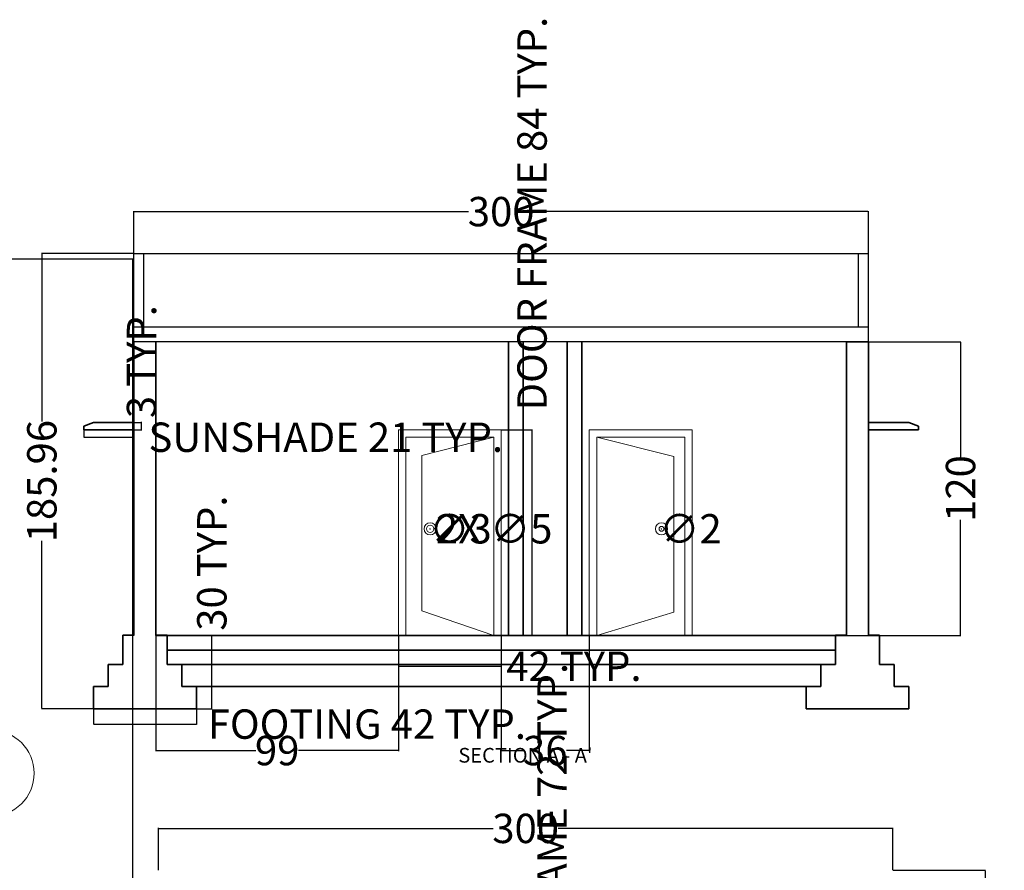
# Model space of a CAD drawing. Units: inches. Extents: x -101 to 786, y 26 to 880.
# Tile 9 of 9: x 379 to 781, y 532 to 879. Entities that reach past the tile are written whole.
import ezdxf

# ---------------------------------------------------------------- set-up
doc = ezdxf.new("R2010")
doc.units = ezdxf.units.IN
doc.header["$MEASUREMENT"] = 0
for name, color, linetype, lineweight in [('A-ANNO-DIMS', 2, 'Continuous', 18), ('A-ANNO-SYMB', 2, 'Continuous', 18), ('A-ANNO-TEXT', 7, 'Continuous', 25), ('A-DOOR', 4, 'Continuous', 20), ('A-ROOF', 7, 'Continuous', 30), ('A-SECT', 7, 'Continuous', 35), ('S-FNDN', 7, 'Continuous', 35)]:
    doc.layers.add(name, color=color, linetype=linetype, lineweight=lineweight)
doc.styles.get("Standard").update_dxf_attribs({"font": 'arial.ttf'})
doc.dimstyles.get("Standard").update_dxf_attribs({"dimtxt": 12, "dimasz": 0.18, "dimexe": 0.18, "dimexo": 0.0625, "dimgap": 0.09, "dimtad": 0, "dimdec": 1, "dimzin": 0, "dimdsep": 46, "dimlunit": 3, "dimtxsty": 'Standard', "dimcen": 0.09, "dimadec": 0, "dimazin": 0, "dimtfac": 1, "dimtdec": 1, "dimtofl": 0, "dimtmove": 0, "dimatfit": 3, "dimfxl": 1, "dimtolj": 1, "dimtzin": 0, "dimarcsym": 0})

# ---------------------------------------------------------------- blocks, each defined once
blk = doc.blocks.new('SUNSHADE-SECTION')
for p, q in [((0, 1.5), (4, 3)), ((0, 0), (0, 1.5)), ((20.5, 3), (4, 3)), ((4, 0), (0, 0)), ((20.5, 0), (4, 0))]:
    blk.add_line(p, q)
blk = doc.blocks.new('FOOTING-STEPPED-42')
for p, q in [((12, 30), (12, 18)), ((16.5, 30), (12, 30)), ((30, 30), (25.5, 30)), ((30, 18), (30, 30)), ((12, 18), (6, 18)), ((6, 18), (6, 9)), ((36, 18), (30, 18)), ((36, 9), (36, 18)), ((6, 9), (0, 9)), ((0, 9), (0, 0)), ((42, 9), (36, 9)), ((42, 0), (42, 9)), ((0, 0), (42, 0))]:
    blk.add_line(p, q)
blk = doc.blocks.new('DOOR-FRAME-36x84-SECT')
blk.add_line((0, 84), (42, 84))
for points in [[(42, 0), (42, 84), (0, 84), (0, 0)], [(39, 0), (39, 81), (3, 81), (3, 0)]]:
    blk.add_lwpolyline(points)
blk = doc.blocks.new('*D45')
at = {"layer": 'A-ANNO-DIMS', "color": 0, "lineweight": -2, "transparency": 16777216}
for p, q in [((404.81, 711.9), (404.81, 708.7)), ((425.31, 711.9), (425.31, 708.7)), ((404.99, 708.88), (425.13, 708.88)), ((425.31, 708.88), (425.49, 708.88))]:
    blk.add_line(p, q, dxfattribs=at)
at = {"layer": 'A-ANNO-DIMS', "color": 0, "transparency": 16777216}
for points in [[(404.99, 708.91), (404.99, 708.85), (404.81, 708.88)], [(425.13, 708.91), (425.13, 708.85), (425.31, 708.88)]]:
    blk.add_solid(points, dxfattribs=at)
at = {"layer": 'Defpoints', "color": 0, "transparency": 16777216}
for p in [(404.81, 711.96), (425.31, 711.96), (425.31, 708.88)]:
    blk.add_point(p, dxfattribs=at)
at = {"layer": 'A-ANNO-DIMS', "color": 0, "transparency": 16777216, "insert": (503.66, 708.88), "char_height": 12, "attachment_point": 5}
blk.add_mtext('\\A1;SUNSHADE 21 TYP.', dxfattribs=at)
blk = doc.blocks.new('*D46')
at = {"layer": 'A-ANNO-DIMS', "color": 0, "lineweight": -2, "transparency": 16777216}
for p, q in [((425.37, 714.96), (428.57, 714.96)), ((425.37, 711.96), (428.57, 711.96)), ((428.39, 714.96), (428.39, 715.14)), ((428.39, 712.14), (428.39, 714.78))]:
    blk.add_line(p, q, dxfattribs=at)
at = {"layer": 'A-ANNO-DIMS', "color": 0, "transparency": 16777216}
for points in [[(428.36, 714.78), (428.42, 714.78), (428.39, 714.96)], [(428.36, 712.14), (428.42, 712.14), (428.39, 711.96)]]:
    blk.add_solid(points, dxfattribs=at)
at = {"layer": 'Defpoints', "color": 0, "transparency": 16777216}
for p in [(425.31, 714.96), (425.31, 711.96), (428.39, 714.96)]:
    blk.add_point(p, dxfattribs=at)
at = {"layer": 'A-ANNO-DIMS', "color": 0, "transparency": 16777216, "insert": (428.39, 739.77), "char_height": 12, "attachment_point": 5, "rotation": 90}
blk.add_mtext('\\A1;3 TYP.', dxfattribs=at)
blk = doc.blocks.new('*D53')
at = {"layer": 'A-ANNO-DIMS', "color": 0, "lineweight": -2, "transparency": 16777216}
for p, q in [((408.81, 597.9), (408.81, 591.48)), ((450.81, 597.9), (450.81, 591.48)), ((408.99, 591.66), (450.63, 591.66)), ((450.81, 591.66), (450.99, 591.66))]:
    blk.add_line(p, q, dxfattribs=at)
at = {"layer": 'A-ANNO-DIMS', "color": 0, "transparency": 16777216}
for points in [[(408.99, 591.69), (408.99, 591.63), (408.81, 591.66)], [(450.63, 591.69), (450.63, 591.63), (450.81, 591.66)]]:
    blk.add_solid(points, dxfattribs=at)
at = {"layer": 'Defpoints', "color": 0, "transparency": 16777216}
for p in [(408.81, 597.96), (450.81, 597.96), (450.81, 591.66)]:
    blk.add_point(p, dxfattribs=at)
at = {"layer": 'A-ANNO-DIMS', "color": 0, "transparency": 16777216, "insert": (520.45, 591.66), "char_height": 12, "attachment_point": 5}
blk.add_mtext('\\A1;FOOTING 42 TYP.', dxfattribs=at)
blk = doc.blocks.new('*D54')
at = {"layer": 'A-ANNO-DIMS', "color": 0, "lineweight": -2, "transparency": 16777216}
for p, q in [((450.87, 627.96), (457.29, 627.96)), ((457.11, 627.96), (457.11, 628.14)), ((457.11, 598.14), (457.11, 627.78)), ((450.87, 597.96), (457.29, 597.96))]:
    blk.add_line(p, q, dxfattribs=at)
at = {"layer": 'A-ANNO-DIMS', "color": 0, "transparency": 16777216}
for points in [[(457.08, 627.78), (457.14, 627.78), (457.11, 627.96)], [(457.08, 598.14), (457.14, 598.14), (457.11, 597.96)]]:
    blk.add_solid(points, dxfattribs=at)
at = {"layer": 'Defpoints', "color": 0, "transparency": 16777216}
for p in [(450.81, 627.96), (457.11, 627.96), (450.81, 597.96)]:
    blk.add_point(p, dxfattribs=at)
at = {"layer": 'A-ANNO-DIMS', "color": 0, "transparency": 16777216, "insert": (457.11, 657.43), "char_height": 12, "attachment_point": 5, "rotation": 90}
blk.add_mtext('\\A1;30 TYP.', dxfattribs=at)
blk = doc.blocks.new('*D61')
at = {"layer": 'A-ANNO-DIMS', "color": 0, "lineweight": -2, "transparency": 16777216}
for p, q in [((575.37, 711.92), (588.09, 711.92)), ((587.91, 711.92), (587.91, 712.1)), ((587.91, 628.1), (587.91, 711.74)), ((575.37, 627.92), (588.09, 627.92))]:
    blk.add_line(p, q, dxfattribs=at)
at = {"layer": 'A-ANNO-DIMS', "color": 0, "transparency": 16777216}
for points in [[(587.88, 711.74), (587.94, 711.74), (587.91, 711.92)], [(587.88, 628.1), (587.94, 628.1), (587.91, 627.92)]]:
    blk.add_solid(points, dxfattribs=at)
at = {"layer": 'Defpoints', "color": 0, "transparency": 16777216}
for p in [(575.31, 711.92), (587.91, 711.92), (575.31, 627.92)]:
    blk.add_point(p, dxfattribs=at)
at = {"layer": 'A-ANNO-DIMS', "color": 0, "transparency": 16777216, "insert": (587.91, 800.24), "char_height": 12, "attachment_point": 5, "rotation": 90}
blk.add_mtext('\\A1;DOOR FRAME 84 TYP.', dxfattribs=at)
blk = doc.blocks.new('*D62')
at = {"layer": 'A-ANNO-DIMS', "color": 0, "lineweight": -2, "transparency": 16777216}
for p, q in [((533.31, 627.86), (533.31, 615.14)), ((575.31, 627.86), (575.31, 615.14)), ((533.49, 615.32), (575.13, 615.32)), ((575.31, 615.32), (575.49, 615.32))]:
    blk.add_line(p, q, dxfattribs=at)
at = {"layer": 'A-ANNO-DIMS', "color": 0, "transparency": 16777216}
for points in [[(533.49, 615.35), (533.49, 615.29), (533.31, 615.32)], [(575.13, 615.35), (575.13, 615.29), (575.31, 615.32)]]:
    blk.add_solid(points, dxfattribs=at)
at = {"layer": 'Defpoints', "color": 0, "transparency": 16777216}
for p in [(533.31, 627.92), (575.31, 627.92), (575.31, 615.32)]:
    blk.add_point(p, dxfattribs=at)
at = {"layer": 'A-ANNO-DIMS', "color": 0, "transparency": 16777216, "insert": (605.03, 615.32), "char_height": 12, "attachment_point": 5}
blk.add_mtext('\\A1;42 TYP.', dxfattribs=at)
blk = doc.blocks.new('*D63')
at = {"layer": 'A-ANNO-DIMS', "color": 0, "lineweight": -2, "transparency": 16777216}
for p, q in [((585.37, 447.92), (596.29, 447.92)), ((596.11, 447.92), (596.11, 448.1)), ((596.11, 376.1), (596.11, 447.74)), ((585.37, 375.92), (596.29, 375.92))]:
    blk.add_line(p, q, dxfattribs=at)
at = {"layer": 'A-ANNO-DIMS', "color": 0, "transparency": 16777216}
for points in [[(596.08, 447.74), (596.14, 447.74), (596.11, 447.92)], [(596.08, 376.1), (596.14, 376.1), (596.11, 375.92)]]:
    blk.add_solid(points, dxfattribs=at)
at = {"layer": 'Defpoints', "color": 0, "transparency": 16777216}
for p in [(585.31, 447.92), (596.11, 447.92), (585.31, 375.92)]:
    blk.add_point(p, dxfattribs=at)
at = {"layer": 'A-ANNO-DIMS', "color": 0, "transparency": 16777216, "insert": (596.11, 536.24), "char_height": 12, "attachment_point": 5, "rotation": 90}
blk.add_mtext('\\A1;DOOR FRAME 72 TYP.', dxfattribs=at)
blk = doc.blocks.new('*D80')
at = {"layer": 'A-ANNO-DIMS', "color": 0, "lineweight": -2, "transparency": 16777216}
for p, q in [((323.57, 781.8), (424.94, 781.8)), ((424.76, 781.62), (424.76, 472.49)), ((424.76, 122.52), (424.76, 431.66)), ((323.57, 122.34), (424.94, 122.34))]:
    blk.add_line(p, q, dxfattribs=at)
at = {"layer": 'A-ANNO-DIMS', "color": 0, "transparency": 16777216}
for points in [[(424.73, 781.62), (424.79, 781.62), (424.76, 781.8)], [(424.73, 122.52), (424.79, 122.52), (424.76, 122.34)]]:
    blk.add_solid(points, dxfattribs=at)
at = {"layer": 'Defpoints', "color": 0, "transparency": 16777216}
for p in [(323.51, 781.8), (424.76, 781.8), (323.51, 122.34)]:
    blk.add_point(p, dxfattribs=at)
at = {"layer": 'A-ANNO-DIMS', "color": 0, "transparency": 16777216, "insert": (424.76, 452.07), "char_height": 12, "attachment_point": 5, "rotation": 90}
blk.add_mtext('\\A1;659.5', dxfattribs=at)
blk = doc.blocks.new('*D119')
at = {"layer": 'A-ANNO-DIMS', "color": 0, "lineweight": -2, "transparency": 16777216}
for p, q in [((425.31, 783.99), (425.31, 801.23)), ((425.49, 801.05), (561.99, 801.05)), ((725.13, 801.05), (588.63, 801.05)), ((725.31, 783.99), (725.31, 801.23))]:
    blk.add_line(p, q, dxfattribs=at)
at = {"layer": 'A-ANNO-DIMS', "color": 0, "transparency": 16777216}
for points in [[(425.49, 801.08), (425.49, 801.02), (425.31, 801.05)], [(725.13, 801.08), (725.13, 801.02), (725.31, 801.05)]]:
    blk.add_solid(points, dxfattribs=at)
at = {"layer": 'Defpoints', "color": 0, "transparency": 16777216}
for p in [(725.31, 801.05), (425.31, 783.92), (725.31, 783.92)]:
    blk.add_point(p, dxfattribs=at)
at = {"layer": 'A-ANNO-DIMS', "color": 0, "transparency": 16777216, "insert": (575.31, 801.05), "char_height": 12, "attachment_point": 5}
blk.add_mtext('\\A1;300', dxfattribs=at)
blk = doc.blocks.new('*D120')
at = {"layer": 'A-ANNO-DIMS', "color": 0, "lineweight": -2, "transparency": 16777216}
for p, q in [((425.25, 783.92), (387.5, 783.92)), ((387.68, 783.74), (387.68, 715.37)), ((387.68, 598.14), (387.68, 666.51)), ((408.74, 597.96), (387.5, 597.96))]:
    blk.add_line(p, q, dxfattribs=at)
at = {"layer": 'A-ANNO-DIMS', "color": 0, "transparency": 16777216}
for points in [[(387.65, 783.74), (387.71, 783.74), (387.68, 783.92)], [(387.65, 598.14), (387.71, 598.14), (387.68, 597.96)]]:
    blk.add_solid(points, dxfattribs=at)
at = {"layer": 'Defpoints', "color": 0, "transparency": 16777216}
for p in [(387.68, 783.92), (425.31, 783.92), (408.81, 597.96)]:
    blk.add_point(p, dxfattribs=at)
at = {"layer": 'A-ANNO-DIMS', "color": 0, "transparency": 16777216, "insert": (387.68, 690.94), "char_height": 12, "attachment_point": 5, "rotation": 90}
blk.add_mtext('\\A1;185.96', dxfattribs=at)
blk = doc.blocks.new('*D121')
at = {"layer": 'A-ANNO-DIMS', "color": 0, "lineweight": -2, "transparency": 16777216}
for p, q in [((716.37, 747.92), (763.12, 747.92)), ((762.94, 747.74), (762.94, 700.69)), ((762.94, 628.1), (762.94, 675.16)), ((716.37, 627.92), (763.12, 627.92))]:
    blk.add_line(p, q, dxfattribs=at)
at = {"layer": 'A-ANNO-DIMS', "color": 0, "transparency": 16777216}
for points in [[(762.91, 747.74), (762.97, 747.74), (762.94, 747.92)], [(762.91, 628.1), (762.97, 628.1), (762.94, 627.92)]]:
    blk.add_solid(points, dxfattribs=at)
at = {"layer": 'Defpoints', "color": 0, "transparency": 16777216}
for p in [(716.31, 747.92), (762.94, 747.92), (716.31, 627.92)]:
    blk.add_point(p, dxfattribs=at)
at = {"layer": 'A-ANNO-DIMS', "color": 0, "transparency": 16777216, "insert": (762.94, 687.92), "char_height": 12, "attachment_point": 5, "rotation": 90}
blk.add_mtext('\\A1;120', dxfattribs=at)
blk = doc.blocks.new('*D122')
at = {"layer": 'A-ANNO-DIMS', "color": 0, "lineweight": -2, "transparency": 16777216}
for p, q in [((434.31, 627.86), (434.31, 580.66)), ((533.31, 627.86), (533.31, 580.66)), ((434.49, 580.84), (475.11, 580.84)), ((533.13, 580.84), (492.51, 580.84))]:
    blk.add_line(p, q, dxfattribs=at)
at = {"layer": 'A-ANNO-DIMS', "color": 0, "transparency": 16777216}
for points in [[(434.49, 580.87), (434.49, 580.81), (434.31, 580.84)], [(533.13, 580.87), (533.13, 580.81), (533.31, 580.84)]]:
    blk.add_solid(points, dxfattribs=at)
at = {"layer": 'Defpoints', "color": 0, "transparency": 16777216}
for p in [(434.31, 627.92), (533.31, 627.92), (533.31, 580.84)]:
    blk.add_point(p, dxfattribs=at)
at = {"layer": 'A-ANNO-DIMS', "color": 0, "transparency": 16777216, "insert": (483.81, 580.84), "char_height": 12, "attachment_point": 5}
blk.add_mtext('\\A1;99', dxfattribs=at)
blk = doc.blocks.new('*D123')
at = {"layer": 'A-ANNO-DIMS', "color": 0, "lineweight": -2, "transparency": 16777216}
for p, q in [((575.31, 627.86), (575.31, 580.66)), ((611.31, 627.86), (611.31, 580.66)), ((575.49, 580.84), (584.64, 580.84)), ((611.13, 580.84), (601.99, 580.84))]:
    blk.add_line(p, q, dxfattribs=at)
at = {"layer": 'A-ANNO-DIMS', "color": 0, "transparency": 16777216}
for points in [[(575.49, 580.87), (575.49, 580.81), (575.31, 580.84)], [(611.13, 580.87), (611.13, 580.81), (611.31, 580.84)]]:
    blk.add_solid(points, dxfattribs=at)
at = {"layer": 'Defpoints', "color": 0, "transparency": 16777216}
for p in [(575.31, 627.92), (611.31, 627.92), (611.31, 580.84)]:
    blk.add_point(p, dxfattribs=at)
at = {"layer": 'A-ANNO-DIMS', "color": 0, "transparency": 16777216, "insert": (593.31, 580.84), "char_height": 12, "attachment_point": 5}
blk.add_mtext('\\A1;36', dxfattribs=at)
blk = doc.blocks.new('*D124')
at = {"layer": 'A-ANNO-DIMS', "color": 0, "lineweight": -2, "transparency": 16777216}
for p, q in [((435.31, 531.99), (435.31, 549.23)), ((435.49, 549.05), (571.99, 549.05)), ((735.13, 549.05), (598.63, 549.05)), ((735.31, 531.99), (735.31, 549.23))]:
    blk.add_line(p, q, dxfattribs=at)
at = {"layer": 'A-ANNO-DIMS', "color": 0, "transparency": 16777216}
for points in [[(435.49, 549.08), (435.49, 549.02), (435.31, 549.05)], [(735.13, 549.08), (735.13, 549.02), (735.31, 549.05)]]:
    blk.add_solid(points, dxfattribs=at)
at = {"layer": 'Defpoints', "color": 0, "transparency": 16777216}
for p in [(735.31, 549.05), (435.31, 531.92), (735.31, 531.92)]:
    blk.add_point(p, dxfattribs=at)
at = {"layer": 'A-ANNO-DIMS', "color": 0, "transparency": 16777216, "insert": (585.31, 549.05), "char_height": 12, "attachment_point": 5}
blk.add_mtext('\\A1;300', dxfattribs=at)
blk = doc.blocks.new('*D125')
at = {"layer": 'A-ANNO-DIMS', "color": 0, "lineweight": -2, "transparency": 16777216}
for p, q in [((735.37, 531.92), (773.12, 531.92)), ((772.94, 531.74), (772.94, 463.37)), ((772.94, 346.14), (772.94, 414.51)), ((751.88, 345.96), (773.12, 345.96))]:
    blk.add_line(p, q, dxfattribs=at)
at = {"layer": 'A-ANNO-DIMS', "color": 0, "transparency": 16777216}
for points in [[(772.91, 531.74), (772.97, 531.74), (772.94, 531.92)], [(772.91, 346.14), (772.97, 346.14), (772.94, 345.96)]]:
    blk.add_solid(points, dxfattribs=at)
at = {"layer": 'Defpoints', "color": 0, "transparency": 16777216}
for p in [(735.31, 531.92), (772.94, 531.92), (751.82, 345.96)]:
    blk.add_point(p, dxfattribs=at)
at = {"layer": 'A-ANNO-DIMS', "color": 0, "transparency": 16777216, "insert": (772.94, 438.94), "char_height": 12, "attachment_point": 5, "rotation": 90}
blk.add_mtext('\\A1;185.96', dxfattribs=at)
blk = doc.blocks.new('*D136')
at = {"layer": 'A-ANNO-DIMS', "color": 0, "lineweight": -2, "transparency": 16777216}
for p, q in [((546.22, 671.46), (546.4, 671.46)), ((546.31, 671.37), (546.31, 671.55)), ((549.17, 671.46), (548.99, 671.46))]:
    blk.add_line(p, q, dxfattribs=at)
at = {"layer": 'A-ANNO-DIMS', "color": 0, "transparency": 16777216}
blk.add_solid([(548.99, 671.49), (548.99, 671.43), (548.81, 671.46)], dxfattribs=at)
at = {"layer": 'Defpoints', "color": 0, "transparency": 16777216}
for p in [(543.81, 671.46), (548.81, 671.46)]:
    blk.add_point(p, dxfattribs=at)
at = {"layer": 'A-ANNO-DIMS', "color": 0, "transparency": 16777216, "insert": (572.44, 671.46), "char_height": 12, "attachment_point": 5, "rotation": 0.0081}
blk.add_mtext('\\A1;2X ∅5', dxfattribs=at)
blk = doc.blocks.new('*D137')
at = {"layer": 'A-ANNO-DIMS', "color": 0, "lineweight": -2, "transparency": 16777216}
for p, q in [((546.22, 671.46), (546.4, 671.46)), ((546.31, 671.37), (546.31, 671.55)), ((548.17, 671.46), (547.99, 671.46))]:
    blk.add_line(p, q, dxfattribs=at)
at = {"layer": 'A-ANNO-DIMS', "color": 0, "transparency": 16777216}
blk.add_solid([(547.99, 671.49), (547.99, 671.43), (547.81, 671.46)], dxfattribs=at)
at = {"layer": 'Defpoints', "color": 0, "transparency": 16777216}
for p in [(544.81, 671.46), (547.81, 671.46)]:
    blk.add_point(p, dxfattribs=at)
at = {"layer": 'A-ANNO-DIMS', "color": 0, "transparency": 16777216, "insert": (558.72, 671.46), "char_height": 12, "attachment_point": 5, "rotation": 0.0136}
blk.add_mtext('\\A1;∅3', dxfattribs=at)
blk = doc.blocks.new('*D138')
at = {"layer": 'A-ANNO-DIMS', "color": 0, "lineweight": -2, "transparency": 16777216}
for p, q in [((640.72, 671.46), (640.9, 671.46)), ((640.81, 671.37), (640.81, 671.55)), ((642.17, 671.46), (641.99, 671.46))]:
    blk.add_line(p, q, dxfattribs=at)
at = {"layer": 'A-ANNO-DIMS', "color": 0, "transparency": 16777216}
blk.add_solid([(641.99, 671.49), (641.99, 671.43), (641.81, 671.46)], dxfattribs=at)
at = {"layer": 'Defpoints', "color": 0, "transparency": 16777216}
for p in [(639.81, 671.46), (641.81, 671.46)]:
    blk.add_point(p, dxfattribs=at)
at = {"layer": 'A-ANNO-DIMS', "color": 0, "transparency": 16777216, "insert": (652.66, 671.46), "char_height": 12, "attachment_point": 5, "rotation": 0.0203}
blk.add_mtext('\\A1;∅2', dxfattribs=at)

msp = doc.modelspace()

# ---------------------------------------------------------------- linework, layer by layer
at = {"layer": 'A-ANNO-SYMB'}
msp.add_circle((366.8306, 571.5872), 17.6773, dxfattribs=at)
at = {"layer": 'A-DOOR'}
for p, q in [((572.3117, 708.9238), (542.8583, 701.3432)), ((614.3117, 708.9238), (645.8069, 700.9606)), ((542.8583, 701.3432), (542.8583, 637.9606)), ((645.8069, 700.9606), (645.8069, 637.4606)), ((542.8583, 637.9606), (572.3117, 627.9238)), ((645.8069, 637.4606), (614.3117, 627.9238))]:
    msp.add_line(p, q, dxfattribs=at)
for centre, radius in [((546.3069, 671.4606), 2.5), ((546.3069, 671.4606), 1.5), ((640.8069, 671.4606), 2.5), ((640.8069, 671.4606), 2.5), ((640.8069, 671.4606), 2.5), ((640.8069, 671.4606), 2.5), ((640.8069, 671.4606), 1)]:
    msp.add_circle(centre, radius, dxfattribs=at)
at = {"layer": 'A-ROOF'}
for p, q in [((425.3117, 783.9238), (725.3117, 783.9238)), ((425.3117, 747.9238), (425.3117, 783.9238)), ((429.3117, 753.9238), (429.3117, 783.9238)), ((721.3117, 753.9238), (721.3117, 783.9238)), ((725.3117, 747.9238), (725.3117, 783.9238)), ((425.3117, 753.9238), (725.3117, 753.9238)), ((425.3117, 747.9238), (725.3117, 747.9238))]:
    msp.add_line(p, q, dxfattribs=at)
at = {"layer": 'A-SECT'}
for p, q in [((425.3117, 627.9238), (425.3117, 747.9238)), ((434.3117, 627.9238), (434.3117, 747.9238)), ((578.3117, 627.9238), (578.3117, 747.9238)), ((584.3117, 627.9238), (584.3117, 747.9238)), ((602.3117, 627.9238), (602.3117, 747.9238)), ((608.3117, 627.9238), (608.3117, 747.9238)), ((716.3117, 627.9238), (716.3117, 747.9238)), ((725.3117, 627.9238), (725.3117, 747.9238)), ((434.3117, 627.9238), (716.3117, 627.9238))]:
    msp.add_line(p, q, dxfattribs=at)
at = {"layer": 'S-FNDN'}
for p, q in [((438.8069, 621.9238), (711.8166, 621.9238)), ((444.8069, 615.9606), (705.8166, 615.9606)), ((450.8069, 606.9606), (699.8166, 606.9606))]:
    msp.add_line(p, q, dxfattribs=at)

# ---------------------------------------------------------------- block references
at = {"layer": 'A-DOOR'}
for p in [(533.312, 627.924), (611.312, 627.924)]:
    msp.add_blockref('DOOR-FRAME-36x84-SECT', p, dxfattribs=at)
at = {"layer": 'A-SECT'}
msp.add_blockref('SUNSHADE-SECTION', (404.807, 711.961), dxfattribs=at)
at = {"layer": 'A-SECT', "extrusion": (0, 0, -1), "zscale": -1}
msp.add_blockref('SUNSHADE-SECTION', (-745.8165, 711.961), dxfattribs=at)
at = {"layer": 'S-FNDN'}
msp.add_blockref('FOOTING-STEPPED-42', (408.807, 597.961), dxfattribs=at)
at = {"layer": 'S-FNDN', "extrusion": (0, 0, -1), "zscale": -1}
msp.add_blockref('FOOTING-STEPPED-42', (-741.8165, 597.961), dxfattribs=at)

# ---------------------------------------------------------------- texts
at = {"layer": 'A-ANNO-TEXT'}
msp.add_text("SECTION A - A'", height=6, dxfattribs=at).set_placement((557.8117, 575.9238))

# ---------------------------------------------------------------- dimensions: what is measured, and where the dimension line sits
at = {"layer": 'A-ANNO-DIMS'}
for base, p1, p2, text, picture, middle in [((587.9117, 711.9238), (575.3117, 627.9238), (575.3117, 711.9238), 'DOOR FRAME <> TYP.', '*D61', (587.9117, 800.2415)), ((428.3875, 714.9606), (425.3117, 711.9606), (425.3117, 714.9606), '<> TYP.', '*D46', (428.3875, 739.7709)), ((457.1069, 627.9606), (450.8069, 597.9606), (450.8069, 627.9606), '<> TYP.', '*D54', (457.1069, 657.4326)), ((596.1117, 447.9238), (585.3117, 375.9238), (585.3117, 447.9238), 'DOOR FRAME <> TYP.', '*D63', (596.1117, 536.2415))]:
    dim = msp.add_linear_dim(base=base, p1=p1, p2=p2, angle=90, text=text, dimstyle='Standard', override={"dimdec": 0, "dimlfac": 1, "dimrnd": 0, "dimzin": 0, "dimdsep": 46, "dimlunit": 2}, dxfattribs=at)
    dim.commit()
    dim.dimension.update_dxf_attribs({"geometry": picture, "text_midpoint": middle})
for base, p1, p2, picture, middle in [((725.3117, 801.0488), (425.3117, 783.9238), (725.3117, 783.9238), '*D119', (575.3117, 801.0488)), ((533.3117, 580.8356), (434.3117, 627.9238), (533.3117, 627.9238), '*D122', (483.8117, 580.8356)), ((611.3117, 580.8356), (575.3117, 627.9238), (611.3117, 627.9238), '*D123', (593.3117, 580.8356)), ((735.3117, 549.0488), (435.3117, 531.9238), (735.3117, 531.9238), '*D124', (585.3117, 549.0488))]:
    dim = msp.add_linear_dim(base=base, p1=p1, p2=p2, dimstyle='Standard', override={"dimdec": 0, "dimlfac": 1, "dimrnd": 0, "dimzin": 0, "dimdsep": 46, "dimlunit": 2}, dxfattribs=at)
    dim.commit()
    dim.dimension.update_dxf_attribs({"geometry": picture, "text_midpoint": middle})
for base, p1, p2, override, picture, middle in [((424.7579, 781.8033), (323.5071, 122.3446), (323.5071, 781.8033), {"dimdec": 1, "dimlfac": 1, "dimrnd": 0, "dimzin": 0, "dimdsep": 46, "dimlunit": 2}, '*D80', (424.7579, 452.0739)), ((387.6819, 783.9238), (408.8069, 597.9606), (425.3117, 783.9238), {"dimdec": 2, "dimlfac": 1, "dimrnd": 0, "dimzin": 0, "dimdsep": 46, "dimlunit": 2}, '*D120', (387.6819, 690.9422)), ((762.9416, 747.9238), (716.3117, 627.9238), (716.3117, 747.9238), {"dimdec": 0, "dimlfac": 1, "dimrnd": 0, "dimzin": 0, "dimdsep": 46, "dimlunit": 2}, '*D121', (762.9416, 687.9238)), ((772.9416, 531.9238), (751.8166, 345.9606), (735.3117, 531.9238), {"dimdec": 2, "dimlfac": 1, "dimrnd": 0, "dimzin": 0, "dimdsep": 46, "dimlunit": 2}, '*D125', (772.9416, 438.9422))]:
    dim = msp.add_linear_dim(base=base, p1=p1, p2=p2, angle=90, dimstyle='Standard', override=override, dxfattribs=at)
    dim.commit()
    dim.dimension.update_dxf_attribs({"geometry": picture, "text_midpoint": middle})
for base, p1, p2, text, picture, middle in [((425.3117, 708.8849), (404.8069, 711.9606), (425.3117, 711.9606), 'SUNSHADE <> TYP.', '*D45', (503.6636, 708.8849)), ((575.3117, 615.3238), (533.3117, 627.9238), (575.3117, 627.9238), '<> TYP.', '*D62', (605.0292, 615.3238)), ((450.8069, 591.6606), (408.8069, 597.9606), (450.8069, 597.9606), 'FOOTING <> TYP.', '*D53', (520.4534, 591.6606))]:
    dim = msp.add_linear_dim(base=base, p1=p1, p2=p2, text=text, dimstyle='Standard', override={"dimdec": 0, "dimlfac": 1, "dimrnd": 0, "dimzin": 0, "dimdsep": 46, "dimlunit": 2}, dxfattribs=at)
    dim.commit()
    dim.dimension.update_dxf_attribs({"geometry": picture, "text_midpoint": middle})
dim = msp.add_diameter_dim_2p(p1=(543.8069, 671.4603), p2=(548.8069, 671.461), text='2X <>', dimstyle='Standard', override={"dimdec": 0, "dimlfac": 1, "dimrnd": 0, "dimzin": 0, "dimdsep": 46, "dimlunit": 2}, dxfattribs=at)
dim.commit()
dim.dimension.update_dxf_attribs({"geometry": '*D136', "text_midpoint": (572.4383, 671.4644), "dimtype": 163})
for p1, p2, picture, middle in [((544.8069, 671.4603), (547.8069, 671.461), '*D137', (558.718, 671.4636)), ((639.8069, 671.4603), (641.8069, 671.461), '*D138', (652.6566, 671.4649))]:
    dim = msp.add_diameter_dim_2p(p1=p1, p2=p2, dimstyle='Standard', override={"dimdec": 0, "dimlfac": 1, "dimrnd": 0, "dimzin": 0, "dimdsep": 46, "dimlunit": 2}, dxfattribs=at)
    dim.commit()
    dim.dimension.update_dxf_attribs({"geometry": picture, "text_midpoint": middle})

doc.saveas('drawing.dxf')
